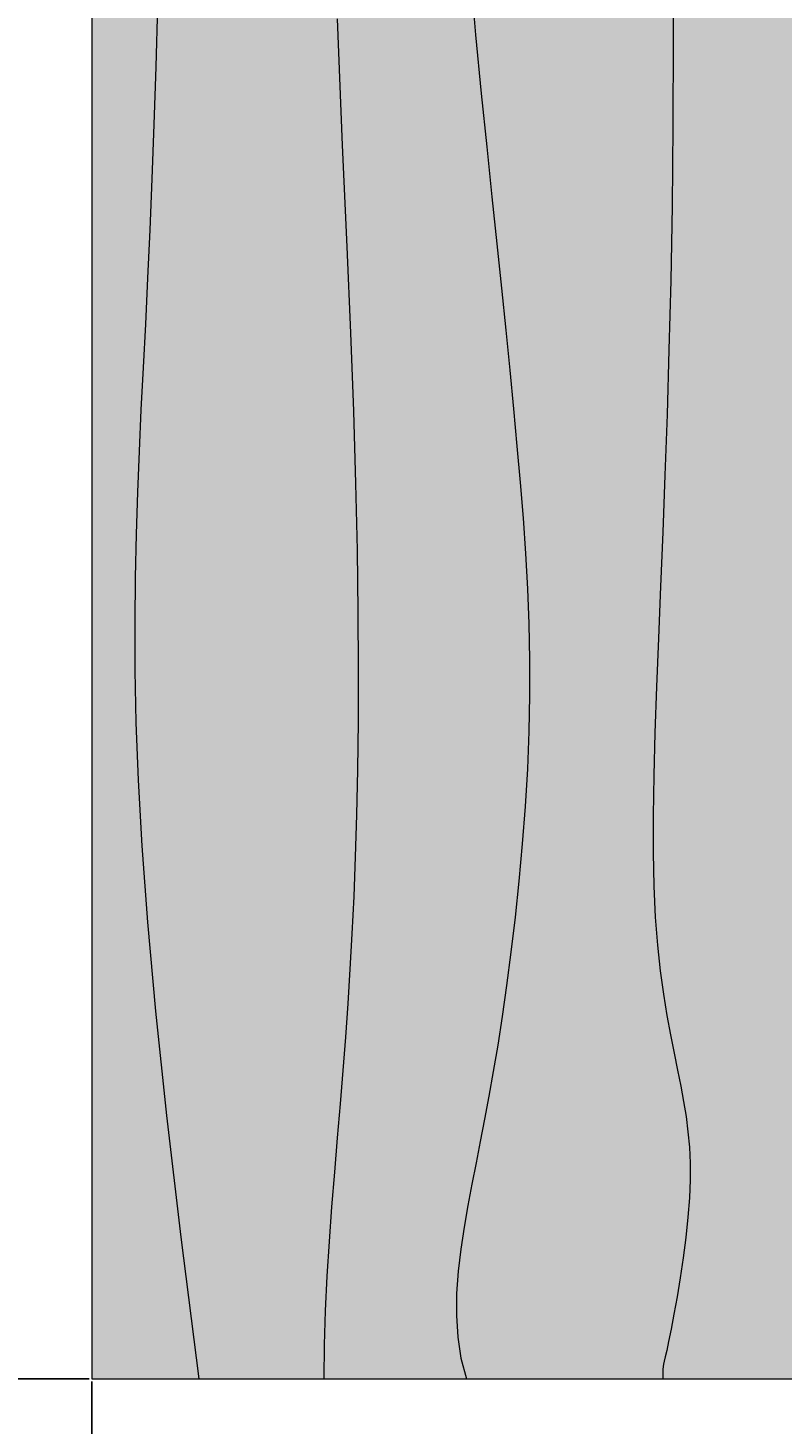
# Model space of a CAD drawing. Units: inches. Extents: x 2549 to 3108, y 1683 to 2362.
# Tile 24 of 30: x 2949 to 2966, y 2018 to 2049. Entities that reach past the tile are written whole.
import ezdxf

# ---------------------------------------------------------------- set-up
doc = ezdxf.new("R2010")
doc.units = ezdxf.units.IN
for name, color, linetype, lineweight in [('A-ANNO-DIMS', 2, 'Continuous', 18), ('A-FURN', 8, 'Continuous', 18), ('A-FURN-PATT', 9, 'Continuous', 13)]:
    doc.layers.add(name, color=color, linetype=linetype, lineweight=lineweight)
doc.layers.add('C-PKNG-VEHI-PATT', color=251, linetype='Continuous', lineweight=13, true_color=0x636466)
doc.layers.add('C-PVMT-PATT', color=9, linetype='Continuous', lineweight=13, true_color=0xc7c8ca)
doc.styles.get("Standard").update_dxf_attribs({"font": 'arial.ttf'})
doc.dimstyles.get("Standard").update_dxf_attribs({"dimtxt": 0.18, "dimasz": 0.18, "dimexe": 0.18, "dimexo": 0.0625, "dimgap": 0.09, "dimtad": 0, "dimtih": 1, "dimtoh": 1, "dimdec": 4, "dimzin": 0, "dimdsep": 46, "dimtxsty": 'Standard', "dimcen": 0.09, "dimadec": 0, "dimazin": 0, "dimtfac": 1, "dimtdec": 4, "dimtofl": 0, "dimtmove": 0, "dimatfit": 3, "dimfxl": 1, "dimtolj": 1, "dimtzin": 0, "dimarcsym": 0})

# ---------------------------------------------------------------- blocks, each defined once
blk = doc.blocks.new('Table - Rectangular Woodgrain 60 x 30 in.')
for p, q in [((60, -30), (60, 0)), ((0, -30), (60, -30))]:
    blk.add_line(p, q)
for points in [[(27.9, -16.9667), (29.9928, -16.9617), (31.9302, -16.9703), (33.7254, -16.9907), (35.3917, -17.0208), (36.9423, -17.0588), (38.3906, -17.1026), (39.7499, -17.1503), (41.0333, -17.2), (42.2519, -17.2496), (43.4073, -17.2969), (44.4986, -17.3395), (45.525, -17.375), (46.4858, -17.4012), (47.3802, -17.4156), (48.2074, -17.416), (48.9667, -17.4), (49.6583, -17.3662), (50.2872, -17.3167), (50.8595, -17.2547), (51.3812, -17.1833), (51.8584, -17.1057), (52.2971, -17.025), (52.7034, -16.9443), (53.0833, -16.8667), (53.443, -16.7951), (53.789, -16.7313), (54.128, -16.6768), (54.4666, -16.6334), (54.8115, -16.6024), (55.1693, -16.5854), (55.5465, -16.5841), (55.95, -16.6), (56.3828, -16.6337), (56.8346, -16.6823), (57.2915, -16.7418), (57.7396, -16.8084), (58.165, -16.878), (58.5539, -16.9469), (58.8924, -17.0111), (59.1666, -17.0667), (59.3679, -17.1107), (59.5078, -17.1438), (59.6032, -17.1675), (59.6708, -17.1833), (59.7275, -17.193), (59.7901, -17.1979), (59.8753, -17.1998), (60, -17.2)], [(28.2656, -21.5281), (29.884, -21.3947), (31.2, -21.2667), (32.3967, -21.1448), (33.5172, -21.0292), (34.5697, -20.9198), (35.5625, -20.8167), (36.5037, -20.7198), (37.4015, -20.6292), (38.2642, -20.5448), (39.1, -20.4667), (39.9164, -20.3951), (40.7187, -20.3313), (41.5117, -20.2768), (42.3, -20.2333), (43.0883, -20.2024), (43.8812, -20.1854), (44.6836, -20.1841), (45.5, -20.2), (46.3328, -20.234), (47.1747, -20.2844), (48.0163, -20.3488), (48.8479, -20.425), (49.66, -20.5106), (50.4429, -20.6031), (51.1872, -20.7004), (51.8833, -20.8), (52.5246, -20.8999), (53.1166, -20.9995), (53.6681, -21.0983), (54.1875, -21.1958), (54.6834, -21.2919), (55.1646, -21.3859), (55.6394, -21.4777), (56.1167, -21.5667), (56.6028, -21.6515), (57.0961, -21.7266), (57.5929, -21.7852), (58.0896, -21.8208), (58.5823, -21.8268), (59.0674, -21.7964), (59.5412, -21.723), (60, -21.6)], [(29.529, -24.4988), (32.3578, -24.3844), (34.6359, -24.284), (36.5667, -24.2), (38.3213, -24.1341), (39.9417, -24.0854), (41.437, -24.0523), (42.8167, -24.0333), (44.0901, -24.0268), (45.2667, -24.0313), (46.3557, -24.0451), (47.3667, -24.0667), (48.309, -24.0947), (49.1928, -24.1287), (50.0284, -24.168), (50.826, -24.2125), (51.5959, -24.2617), (52.3483, -24.3151), (53.0935, -24.3725), (53.8417, -24.4334), (54.6009, -24.497), (55.3699, -24.561), (56.1454, -24.6226), (56.9239, -24.6792), (57.7021, -24.7279), (58.4764, -24.7662), (59.2435, -24.7911), (60, -24.8)], [(29.2276, -28.5281), (30.6033, -28.5663), (31.8958, -28.6084), (33.1118, -28.6535), (34.2578, -28.7011), (35.3405, -28.7501), (36.3666, -28.8), (37.3443, -28.8497), (38.288, -28.8974), (39.2137, -28.9412), (40.1375, -28.9792), (41.0753, -29.0093), (42.0432, -29.0297), (43.0572, -29.0384), (44.1333, -29.0333), (45.2936, -29.0114), (46.5843, -28.9641), (48.0579, -28.8816), (49.7666, -28.7542), (51.7629, -28.5721), (54.0989, -28.3255), (56.8272, -28.0048), (60, -27.6)]]:
    blk.add_lwpolyline(points)
blk = doc.blocks.new('*D22')
at = {"layer": 'A-ANNO-DIMS', "color": 0, "lineweight": -2, "transparency": 16777216}
for p, q in [((2950.031, 2078.615), (2940.913, 2078.615)), ((2941.093, 2078.435), (2941.093, 2048.798)), ((2941.093, 2018.795), (2941.093, 2048.431)), ((2950.031, 2018.615), (2940.913, 2018.615))]:
    blk.add_line(p, q, dxfattribs=at)
at = {"layer": 'A-ANNO-DIMS', "color": 0, "transparency": 16777216}
for points in [[(2941.063, 2078.435), (2941.123, 2078.435), (2941.093, 2078.615)], [(2941.063, 2018.795), (2941.123, 2018.795), (2941.093, 2018.615)]]:
    blk.add_solid(points, dxfattribs=at)
at = {"layer": 'Defpoints', "color": 0, "transparency": 16777216}
for p in [(2950.093, 2078.615), (2941.093, 2018.615), (2950.093, 2018.615)]:
    blk.add_point(p, dxfattribs=at)
at = {"layer": 'A-ANNO-DIMS', "color": 0, "transparency": 16777216, "insert": (2941.093, 2048.615), "char_height": 0.18, "attachment_point": 5}
blk.add_mtext('\\A1;COFFEE TABLE 60', dxfattribs=at)
blk = doc.blocks.new('*D23')
at = {"layer": 'A-ANNO-DIMS', "color": 0, "lineweight": -2, "transparency": 16777216}
for p, q in [((2950.093, 2018.552), (2950.093, 2009.435)), ((2980.093, 2018.552), (2980.093, 2009.435)), ((2950.273, 2009.615), (2964.875, 2009.615)), ((2979.913, 2009.615), (2965.312, 2009.615))]:
    blk.add_line(p, q, dxfattribs=at)
at = {"layer": 'A-ANNO-DIMS', "color": 0, "transparency": 16777216}
for points in [[(2950.273, 2009.645), (2950.273, 2009.585), (2950.093, 2009.615)], [(2979.913, 2009.645), (2979.913, 2009.585), (2980.093, 2009.615)]]:
    blk.add_solid(points, dxfattribs=at)
at = {"layer": 'Defpoints', "color": 0, "transparency": 16777216}
for p in [(2950.093, 2018.615), (2980.093, 2018.615), (2980.093, 2009.615)]:
    blk.add_point(p, dxfattribs=at)
at = {"layer": 'A-ANNO-DIMS', "color": 0, "transparency": 16777216, "insert": (2965.093, 2009.615), "char_height": 0.18, "attachment_point": 5}
blk.add_mtext('\\A1;30', dxfattribs=at)
blk = doc.blocks.new('*D46')
at = {"layer": 'A-ANNO-DIMS', "color": 0, "lineweight": -2, "transparency": 16777216}
for p, q in [((2812.643, 2140.461), (2812.643, 1683.444)), ((3034.643, 2134.461), (3034.643, 1683.444)), ((2812.823, 1683.624), (2923.353, 1683.624)), ((3034.463, 1683.624), (2923.932, 1683.624))]:
    blk.add_line(p, q, dxfattribs=at)
at = {"layer": 'A-ANNO-DIMS', "color": 0, "transparency": 16777216}
for points in [[(2812.823, 1683.654), (2812.823, 1683.594), (2812.643, 1683.624)], [(3034.463, 1683.654), (3034.463, 1683.594), (3034.643, 1683.624)]]:
    blk.add_solid(points, dxfattribs=at)
at = {"layer": 'Defpoints', "color": 0, "transparency": 16777216}
for p in [(2812.643, 2140.524), (3034.643, 2134.524), (3034.643, 1683.624)]:
    blk.add_point(p, dxfattribs=at)
at = {"layer": 'A-ANNO-DIMS', "color": 0, "transparency": 16777216, "insert": (2923.643, 1683.624), "char_height": 0.18, "attachment_point": 5}
blk.add_mtext('\\A1;222', dxfattribs=at)
blk = doc.blocks.new('*D63')
at = {"layer": 'A-ANNO-DIMS', "color": 0, "lineweight": -2, "transparency": 16777216}
for p, q in [((2963.328, 2197.213), (2963.508, 2197.213)), ((2963.508, 2197.213), (2963.508, 2124.675)), ((2963.419, 2003.299), (2963.599, 2003.299)), ((2963.509, 2003.209), (2963.509, 2003.389))]:
    blk.add_line(p, q, dxfattribs=at)
at = {"layer": 'A-ANNO-DIMS', "color": 0, "transparency": 16777216}
blk.add_solid([(2963.538, 2124.675), (2963.478, 2124.675), (2963.508, 2124.495)], dxfattribs=at)
at = {"layer": 'Defpoints', "color": 0, "transparency": 16777216}
for p in [(2963.508, 2124.495), (2963.509, 2003.299)]:
    blk.add_point(p, dxfattribs=at)
at = {"layer": 'A-ANNO-DIMS', "color": 0, "transparency": 16777216, "insert": (2962.654, 2197.213), "char_height": 0.18, "attachment_point": 5}
blk.add_mtext('\\A1;2X R121.2', dxfattribs=at)

msp = doc.modelspace()

# ---------------------------------------------------------------- hatches: boundary and pattern name
at = {"layer": 'A-FURN-PATT', "transparency": 33554684}
h = msp.add_hatch(color=256, dxfattribs=at)
h.dxf.hatch_style = 1
h.paths.add_polyline_path([(2951.6587, 2056.0021), (2951.6557, 2058.2435), (2951.6347, 2060.9396), (2951.5919, 2064.2076), (2951.5233, 2068.1646), (2951.425, 2072.9279), (2951.2931, 2078.6146), (2950.0931, 2078.6146), (2950.0931, 2018.6146), (2952.4931, 2018.6146), (2952.0883, 2021.7874), (2951.7676, 2024.5157), (2951.521, 2026.8517), (2951.3389, 2028.848), (2951.2115, 2030.5567), (2951.129, 2032.0303), (2951.0817, 2033.321), (2951.0598, 2034.4813), (2951.0547, 2035.5574), (2951.0634, 2036.5714), (2951.0838, 2037.5393), (2951.1139, 2038.4771), (2951.1519, 2039.4009), (2951.1957, 2040.3266), (2951.2434, 2041.2703), (2951.2931, 2042.248), (2951.343, 2043.2741), (2951.392, 2044.3568), (2951.4396, 2045.5028), (2951.4847, 2046.7188), (2951.5268, 2048.0113), (2951.565, 2049.387), (2951.5984, 2050.8526), (2951.6264, 2052.4146), (2951.6476, 2054.0982)])
h.paths.add_polyline_path([(2955.3325, 2057.2097), (2955.19, 2062.912), (2955.0427, 2069.9791), (2954.8931, 2078.6146), (2951.2931, 2078.6146), (2951.425, 2072.9279), (2951.5233, 2068.1646), (2951.5919, 2064.2076), (2951.6347, 2060.9396), (2951.6557, 2058.2435), (2951.6587, 2056.0021), (2951.6476, 2054.0982), (2951.6264, 2052.4146), (2951.5984, 2050.8526), (2951.565, 2049.387), (2951.5268, 2048.0113), (2951.4847, 2046.7188), (2951.4396, 2045.5028), (2951.392, 2044.3568), (2951.343, 2043.2741), (2951.2931, 2042.248), (2951.2434, 2041.2703), (2951.1957, 2040.3266), (2951.1519, 2039.4009), (2951.1139, 2038.4771), (2951.0838, 2037.5393), (2951.0634, 2036.5714), (2951.0547, 2035.5574), (2951.0598, 2034.4813), (2951.0817, 2033.321), (2951.129, 2032.0303), (2951.2115, 2030.5567), (2951.3389, 2028.848), (2951.521, 2026.8517), (2951.7676, 2024.5157), (2952.0883, 2021.7874), (2952.4931, 2018.6146), (2955.2931, 2018.6146), (2955.302, 2019.3711), (2955.3269, 2020.1382), (2955.3652, 2020.9125), (2955.4139, 2021.6907), (2955.4705, 2022.4692), (2955.5321, 2023.2447), (2955.5961, 2024.0137), (2955.6597, 2024.7729), (2955.7206, 2025.5211), (2955.778, 2026.2663), (2955.8314, 2027.0187), (2955.8806, 2027.7886), (2955.9251, 2028.5862), (2955.9644, 2029.4218), (2955.9984, 2030.3056), (2956.0264, 2031.2479), (2956.048, 2032.2589), (2956.0618, 2033.3479), (2956.0663, 2034.5245), (2956.0598, 2035.7979), (2956.0408, 2037.1776), (2956.0077, 2038.6729), (2955.959, 2040.2933), (2955.8931, 2042.0479), (2955.8091, 2043.9787), (2955.7087, 2046.2568), (2955.5943, 2049.0856), (2955.4681, 2052.6688)])
h.paths.add_polyline_path([(2958.1396, 2059.1978), (2957.992, 2064.2052), (2957.843, 2070.6048), (2957.6931, 2078.6146), (2954.8931, 2078.6146), (2955.0427, 2069.9791), (2955.19, 2062.912), (2955.3325, 2057.2097), (2955.4681, 2052.6688), (2955.5943, 2049.0856), (2955.7087, 2046.2568), (2955.8091, 2043.9787), (2955.8931, 2042.0479), (2955.959, 2040.2933), (2956.0077, 2038.6729), (2956.0408, 2037.1776), (2956.0598, 2035.7979), (2956.0663, 2034.5245), (2956.0618, 2033.3479), (2956.048, 2032.2589), (2956.0264, 2031.2479), (2955.9984, 2030.3056), (2955.9644, 2029.4218), (2955.9251, 2028.5862), (2955.8806, 2027.7886), (2955.8314, 2027.0187), (2955.778, 2026.2663), (2955.7206, 2025.5211), (2955.6597, 2024.7729), (2955.5961, 2024.0137), (2955.5321, 2023.2447), (2955.4705, 2022.4692), (2955.4139, 2021.6907), (2955.3652, 2020.9125), (2955.3269, 2020.1382), (2955.302, 2019.3711), (2955.2931, 2018.6146), (2958.4931, 2018.6146), (2958.3701, 2019.0734), (2958.2967, 2019.5472), (2958.2663, 2020.0323), (2958.2723, 2020.525), (2958.3079, 2021.0217), (2958.3665, 2021.5185), (2958.4416, 2022.0118), (2958.5264, 2022.4979), (2958.6154, 2022.9752), (2958.7072, 2023.45), (2958.8012, 2023.9312), (2958.8973, 2024.4271), (2958.9948, 2024.9465), (2959.0936, 2025.498), (2959.1932, 2026.09), (2959.2931, 2026.7313), (2959.3927, 2027.4274), (2959.49, 2028.1717), (2959.5825, 2028.9546), (2959.6681, 2029.7667), (2959.7443, 2030.5983), (2959.8087, 2031.4399), (2959.8591, 2032.2818), (2959.8931, 2033.1146), (2959.909, 2033.931), (2959.9077, 2034.7334), (2959.8907, 2035.5263), (2959.8598, 2036.3146), (2959.8163, 2037.1029), (2959.7618, 2037.8959), (2959.698, 2038.6982), (2959.6264, 2039.5146), (2959.5483, 2040.3504), (2959.4639, 2041.2131), (2959.3733, 2042.1109), (2959.2764, 2043.0521), (2959.1733, 2044.0449), (2959.0639, 2045.0974), (2958.9483, 2046.2179), (2958.8264, 2047.4146), (2958.6984, 2048.7306), (2958.565, 2050.349), (2958.4268, 2052.4877), (2958.2848, 2055.3646)])
h.paths.add_polyline_path([(2963.0634, 2055.4818), (2962.9958, 2058.2679), (2962.8973, 2061.4021), (2962.7628, 2064.9441), (2962.5874, 2068.9537), (2962.3658, 2073.4906), (2962.0931, 2078.6146), (2957.6931, 2078.6146), (2957.843, 2070.6048), (2957.992, 2064.2052), (2958.1396, 2059.1978), (2958.2848, 2055.3646), (2958.4268, 2052.4877), (2958.565, 2050.349), (2958.6984, 2048.7306), (2958.8264, 2047.4146), (2958.9483, 2046.2179), (2959.0639, 2045.0974), (2959.1733, 2044.0449), (2959.2764, 2043.0521), (2959.3733, 2042.1109), (2959.4639, 2041.2131), (2959.5483, 2040.3504), (2959.6264, 2039.5146), (2959.698, 2038.6982), (2959.7618, 2037.8959), (2959.8163, 2037.1029), (2959.8598, 2036.3146), (2959.8907, 2035.5263), (2959.9077, 2034.7334), (2959.909, 2033.931), (2959.8931, 2033.1146), (2959.8591, 2032.2818), (2959.8087, 2031.4399), (2959.7443, 2030.5983), (2959.6681, 2029.7667), (2959.5825, 2028.9546), (2959.49, 2028.1717), (2959.3927, 2027.4274), (2959.2931, 2026.7313), (2959.1932, 2026.09), (2959.0936, 2025.498), (2958.9948, 2024.9465), (2958.8973, 2024.4271), (2958.8012, 2023.9312), (2958.7072, 2023.45), (2958.6154, 2022.9752), (2958.5264, 2022.4979), (2958.4416, 2022.0118), (2958.3665, 2021.5185), (2958.3079, 2021.0217), (2958.2723, 2020.525), (2958.2663, 2020.0323), (2958.2967, 2019.5472), (2958.3701, 2019.0734), (2958.4931, 2018.6146), (2962.8931, 2018.6146), (2962.8935, 2018.8741), (2962.9256, 2019.0114), (2962.9493, 2019.1068), (2962.9824, 2019.2467), (2963.0264, 2019.448), (2963.082, 2019.7222), (2963.1462, 2020.0607), (2963.2151, 2020.4496), (2963.2847, 2020.875), (2963.3513, 2021.3231), (2963.4108, 2021.78), (2963.4594, 2022.2318), (2963.4931, 2022.6646), (2963.509, 2023.0681), (2963.5077, 2023.4453), (2963.4907, 2023.8031), (2963.4597, 2024.148), (2963.4163, 2024.4866), (2963.3618, 2024.8256), (2963.298, 2025.1716), (2963.2264, 2025.5313), (2963.1488, 2025.9112), (2963.0681, 2026.3175), (2962.9874, 2026.7562), (2962.9098, 2027.2334), (2962.8384, 2027.7551), (2962.7764, 2028.3274), (2962.7269, 2028.9563), (2962.6931, 2029.6479), (2962.6771, 2030.4072), (2962.6775, 2031.2344), (2962.6919, 2032.1288), (2962.7181, 2033.0896), (2962.7536, 2034.116), (2962.7962, 2035.2073), (2962.8435, 2036.3627), (2962.8931, 2037.5813), (2962.9428, 2038.8647), (2962.9905, 2040.224), (2963.0343, 2041.6723), (2963.0723, 2043.2229), (2963.1024, 2044.8892), (2963.1228, 2046.6844), (2963.1314, 2048.6218), (2963.1264, 2050.7146), (2963.1053, 2052.9839)])
h.paths.add_polyline_path([(2967.0608, 2068.9933), (2967.1609, 2073.4299), (2967.2931, 2078.6146), (2962.0931, 2078.6146), (2962.3658, 2073.4906), (2962.5874, 2068.9537), (2962.7628, 2064.9441), (2962.8973, 2061.4021), (2962.9958, 2058.2679), (2963.0634, 2055.4818), (2963.1053, 2052.9839), (2963.1264, 2050.7146), (2963.1314, 2048.6218), (2963.1228, 2046.6844), (2963.1024, 2044.8892), (2963.0723, 2043.2229), (2963.0343, 2041.6723), (2962.9905, 2040.224), (2962.9428, 2038.8647), (2962.8931, 2037.5813), (2962.8435, 2036.3627), (2962.7962, 2035.2073), (2962.7536, 2034.116), (2962.7181, 2033.0896), (2962.6919, 2032.1288), (2962.6775, 2031.2344), (2962.6771, 2030.4072), (2962.6931, 2029.6479), (2962.7269, 2028.9563), (2962.7764, 2028.3274), (2962.8384, 2027.7551), (2962.9098, 2027.2334), (2962.9874, 2026.7562), (2963.0681, 2026.3175), (2963.1488, 2025.9112), (2963.2264, 2025.5313), (2963.298, 2025.1716), (2963.3618, 2024.8256), (2963.4163, 2024.4866), (2963.4597, 2024.148), (2963.4907, 2023.8031), (2963.5077, 2023.4453), (2963.509, 2023.0681), (2963.4931, 2022.6646), (2963.4594, 2022.2318), (2963.4108, 2021.78), (2963.3513, 2021.3231), (2963.2847, 2020.875), (2963.2151, 2020.4496), (2963.1462, 2020.0607), (2963.082, 2019.7222), (2963.0264, 2019.448), (2962.9824, 2019.2467), (2962.9493, 2019.1068), (2962.9256, 2019.0114), (2962.9098, 2018.9438), (2962.9001, 2018.8871), (2962.8952, 2018.8245), (2962.8933, 2018.7393), (2962.8931, 2018.6146), (2966.4931, 2018.6146), (2966.7749, 2019.8457), (2967.0223, 2020.8601), (2967.2384, 2021.6895), (2967.4264, 2022.3657), (2967.5894, 2022.9204), (2967.7306, 2023.3853), (2967.853, 2023.7923), (2967.9598, 2024.173), (2968.0534, 2024.5532), (2968.1337, 2024.9351), (2968.2, 2025.3148), (2968.2514, 2025.6886), (2968.2872, 2026.0526), (2968.3066, 2026.403), (2968.3088, 2026.7361), (2968.2931, 2027.048), (2968.259, 2027.3358), (2968.2077, 2027.6011), (2968.1407, 2027.846), (2968.0598, 2028.073), (2967.9663, 2028.2843), (2967.8618, 2028.4823), (2967.748, 2028.6694), (2967.6264, 2028.8479), (2967.4987, 2029.0209), (2967.367, 2029.1938), (2967.2338, 2029.3729), (2967.1014, 2029.5646), (2966.9721, 2029.775), (2966.8483, 2030.0104), (2966.7323, 2030.2771), (2966.6264, 2030.5813), (2966.5327, 2030.9288), (2966.4514, 2031.324), (2966.3827, 2031.7707), (2966.3264, 2032.273), (2966.2827, 2032.8345), (2966.2514, 2033.4594), (2966.2327, 2034.1515), (2966.2264, 2034.9146), (2966.2324, 2035.7506), (2966.2493, 2036.6521), (2966.2757, 2037.6099), (2966.3098, 2038.6146), (2966.3501, 2039.6568), (2966.3952, 2040.7271), (2966.4434, 2041.8162), (2966.4931, 2042.9146), (2966.543, 2044.0176), (2966.5921, 2045.1386), (2966.6396, 2046.2955), (2966.6848, 2047.5063), (2966.7268, 2048.789), (2966.765, 2050.1615), (2966.7984, 2051.6418), (2966.8264, 2053.248), (2966.8492, 2055.0092), (2966.8712, 2057.0006), (2966.8979, 2059.3083), (2966.9348, 2062.0188), (2966.9872, 2065.2183)])
h.paths.add_polyline_path([(2971.0073, 2072.0387), (2970.8931, 2078.6146), (2967.2931, 2078.6146), (2967.1609, 2073.4299), (2967.0608, 2068.9933), (2966.9872, 2065.2183), (2966.9348, 2062.0188), (2966.8979, 2059.3083), (2966.8712, 2057.0006), (2966.8492, 2055.0092), (2966.8264, 2053.248), (2966.7984, 2051.6418), (2966.765, 2050.1615), (2966.7268, 2048.789), (2966.6848, 2047.5063), (2966.6396, 2046.2955), (2966.5921, 2045.1386), (2966.543, 2044.0176), (2966.4931, 2042.9146), (2966.4434, 2041.8162), (2966.3952, 2040.7271), (2966.3501, 2039.6568), (2966.3098, 2038.6146), (2966.2757, 2037.6099), (2966.2493, 2036.6521), (2966.2324, 2035.7506), (2966.2264, 2034.9146), (2966.2327, 2034.1515), (2966.2514, 2033.4594), (2966.2827, 2032.8345), (2966.3264, 2032.273), (2966.3827, 2031.7707), (2966.4514, 2031.324), (2966.5327, 2030.9288), (2966.6264, 2030.5813), (2966.7323, 2030.2771), (2966.8483, 2030.0104), (2966.9721, 2029.775), (2967.1014, 2029.5646), (2967.2338, 2029.3729), (2967.367, 2029.1938), (2967.4987, 2029.0209), (2967.6264, 2028.8479), (2967.748, 2028.6694), (2967.8618, 2028.4823), (2967.9663, 2028.2843), (2968.0598, 2028.073), (2968.1407, 2027.846), (2968.2077, 2027.6011), (2968.259, 2027.3358), (2968.2931, 2027.048), (2968.3088, 2026.7361), (2968.3066, 2026.403), (2968.2872, 2026.0526), (2968.2514, 2025.6886), (2968.2, 2025.3148), (2968.1337, 2024.9351), (2968.0534, 2024.5532), (2967.9598, 2024.173), (2967.853, 2023.7923), (2967.7306, 2023.3853), (2967.5894, 2022.9204), (2967.4264, 2022.3657), (2967.2384, 2021.6895), (2967.0223, 2020.8601), (2966.7749, 2019.8457), (2966.4931, 2018.6146), (2970.0931, 2018.6146), (2970.5775, 2020.6947), (2971.1181, 2022.524), (2971.6962, 2024.1236), (2972.2931, 2025.5146), (2972.89, 2026.7181), (2973.4681, 2027.7552), (2974.0087, 2028.647), (2974.4931, 2029.4146), (2974.9065, 2030.0774), (2975.2504, 2030.6485), (2975.5302, 2031.139), (2975.7514, 2031.5604), (2975.9195, 2031.924), (2976.04, 2032.2412), (2976.1182, 2032.5231), (2976.1598, 2032.7813), (2976.1697, 2033.0246), (2976.1514, 2033.2532), (2976.1082, 2033.4645), (2976.0431, 2033.6563), (2975.9592, 2033.8262), (2975.8598, 2033.9719), (2975.7478, 2034.091), (2975.6264, 2034.1813), (2975.4975, 2034.241), (2975.3577, 2034.2719), (2975.2022, 2034.2762), (2975.0264, 2034.2563), (2974.8256, 2034.2145), (2974.5952, 2034.1532), (2974.3303, 2034.0746), (2974.0264, 2033.9813), (2973.6814, 2033.8758), (2973.3035, 2033.7625), (2972.9038, 2033.6461), (2972.4931, 2033.5313), (2972.0824, 2033.4227), (2971.6827, 2033.325), (2971.3048, 2033.243), (2970.9598, 2033.1813), (2970.656, 2033.1437), (2970.392, 2033.1302), (2970.1641, 2033.1403), (2969.9681, 2033.173), (2969.8002, 2033.2275), (2969.6566, 2033.3032), (2969.5333, 2033.3991), (2969.4264, 2033.5146), (2969.3328, 2033.6498), (2969.2525, 2033.8084), (2969.1862, 2033.9951), (2969.1348, 2034.2146), (2969.0989, 2034.4716), (2969.0795, 2034.7709), (2969.0773, 2035.117), (2969.0931, 2035.5146), (2969.1271, 2035.9681), (2969.1775, 2036.4802), (2969.2419, 2037.0533), (2969.3181, 2037.6896), (2969.4036, 2038.3916), (2969.4962, 2039.1615), (2969.5935, 2040.0017), (2969.6931, 2040.9146), (2969.7932, 2041.9018), (2969.8941, 2042.962), (2969.9966, 2044.0933), (2970.1014, 2045.2938), (2970.2094, 2046.5614), (2970.3212, 2047.8943), (2970.4378, 2049.2905), (2970.5598, 2050.748), (2970.6862, 2052.2926), (2970.8087, 2054.0615), (2970.9172, 2056.2194), (2971.0014, 2058.9313), (2971.0513, 2062.3619), (2971.0566, 2066.6761)])
h.paths.add_polyline_path([(2977.5454, 2065.9056), (2977.6243, 2069.5844), (2977.6751, 2073.7991), (2977.6931, 2078.6146), (2970.8931, 2078.6146), (2971.0073, 2072.0387), (2971.0566, 2066.6761), (2971.0513, 2062.3619), (2971.0014, 2058.9313), (2970.9172, 2056.2194), (2970.8087, 2054.0615), (2970.6862, 2052.2926), (2970.5598, 2050.748), (2970.4378, 2049.2905), (2970.3212, 2047.8943), (2970.2094, 2046.5614), (2970.1014, 2045.2938), (2969.9966, 2044.0933), (2969.8941, 2042.962), (2969.7932, 2041.9018), (2969.6931, 2040.9146), (2969.5935, 2040.0017), (2969.4962, 2039.1615), (2969.4036, 2038.3916), (2969.3181, 2037.6896), (2969.2419, 2037.0533), (2969.1775, 2036.4802), (2969.1271, 2035.9681), (2969.0931, 2035.5146), (2969.0773, 2035.117), (2969.0795, 2034.7709), (2969.0989, 2034.4716), (2969.1348, 2034.2146), (2969.1862, 2033.9951), (2969.2525, 2033.8084), (2969.3328, 2033.6498), (2969.4264, 2033.5146), (2969.5333, 2033.3991), (2969.6566, 2033.3032), (2969.8002, 2033.2275), (2969.9681, 2033.173), (2970.1641, 2033.1403), (2970.392, 2033.1302), (2970.656, 2033.1437), (2970.9598, 2033.1813), (2971.3048, 2033.243), (2971.6827, 2033.325), (2972.0824, 2033.4227), (2972.4931, 2033.5313), (2972.9038, 2033.6461), (2973.3035, 2033.7625), (2973.6814, 2033.8758), (2974.0264, 2033.9813), (2974.3303, 2034.0746), (2974.5952, 2034.1532), (2974.8256, 2034.2145), (2975.1314, 2034.2781), (2975.4354, 2034.2697), (2975.6264, 2034.1813), (2975.7478, 2034.091), (2975.8598, 2033.9719), (2975.9592, 2033.8262), (2976.0431, 2033.6563), (2976.1082, 2033.4645), (2976.1514, 2033.2532), (2976.1697, 2033.0246), (2976.1598, 2032.7813), (2976.1182, 2032.5231), (2976.04, 2032.2412), (2975.9195, 2031.924), (2975.7514, 2031.5604), (2975.5302, 2031.139), (2975.2504, 2030.6485), (2974.9065, 2030.0774), (2974.4931, 2029.4146), (2974.0087, 2028.647), (2973.4681, 2027.7552), (2972.89, 2026.7181), (2972.2931, 2025.5146), (2971.6962, 2024.1236), (2971.1181, 2022.524), (2970.5775, 2020.6947), (2970.0931, 2018.6146), (2976.8931, 2018.6146), (2977.043, 2020.5019), (2977.192, 2022.3313), (2977.3396, 2024.092), (2977.4848, 2025.773), (2977.6268, 2027.3633), (2977.765, 2028.8521), (2977.8984, 2030.2284), (2978.0264, 2031.4813), (2978.1482, 2032.6032), (2978.2629, 2033.6006), (2978.3698, 2034.483), (2978.4681, 2035.2604), (2978.557, 2035.9425), (2978.6358, 2036.5391), (2978.7036, 2037.0599), (2978.7598, 2037.5146), (2978.8035, 2037.9123), (2978.8348, 2038.2584), (2978.8535, 2038.5576), (2978.8598, 2038.8146), (2978.8535, 2039.0342), (2978.8348, 2039.2209), (2978.8035, 2039.3795), (2978.7598, 2039.5146), (2978.7038, 2039.6302), (2978.6368, 2039.7271), (2978.5605, 2039.8052), (2978.4764, 2039.8646), (2978.3861, 2039.9052), (2978.291, 2039.9271), (2978.1928, 2039.9302), (2978.0931, 2039.9146), (2977.993, 2039.8809), (2977.8921, 2039.8323), (2977.7896, 2039.7728), (2977.6848, 2039.7063), (2977.5003, 2039.5872), (2977.2813, 2039.4666), (2977.0307, 2039.3815), (2976.7627, 2039.3587), (2976.5032, 2039.4189), (2976.3323, 2039.5382), (2976.2264, 2039.648), (2976.1329, 2039.7907), (2976.0535, 2039.9771), (2975.9897, 2040.2198), (2975.9431, 2040.5313), (2975.9152, 2040.924), (2975.9077, 2041.4105), (2975.922, 2042.0032), (2975.9597, 2042.7146), (2976.0217, 2043.5556), (2976.1056, 2044.5297), (2976.2082, 2045.639), (2976.3264, 2046.8855), (2976.4571, 2048.2709), (2976.5973, 2049.7974), (2976.7436, 2051.4669), (2976.8931, 2053.2813), (2977.0423, 2055.253), (2977.1868, 2057.4365), (2977.322, 2059.8965), (2977.4431, 2062.6979)])
h.paths.add_polyline_path([(2980.0931, 2078.6146), (2977.6931, 2078.6146), (2977.6751, 2073.7991), (2977.6243, 2069.5844), (2977.5454, 2065.9056), (2977.4431, 2062.6979), (2977.322, 2059.8965), (2977.1868, 2057.4365), (2977.0423, 2055.253), (2976.8931, 2053.2813), (2976.7436, 2051.4669), (2976.5973, 2049.7974), (2976.4571, 2048.2709), (2976.3264, 2046.8855), (2976.2082, 2045.639), (2976.1056, 2044.5297), (2976.0217, 2043.5556), (2975.9597, 2042.7146), (2975.922, 2042.0032), (2975.9077, 2041.4105), (2975.9152, 2040.924), (2975.9431, 2040.5313), (2975.9897, 2040.2198), (2976.0535, 2039.9771), (2976.1329, 2039.7907), (2976.2264, 2039.648), (2976.3323, 2039.5382), (2976.4483, 2039.4573), (2976.5721, 2039.403), (2976.7014, 2039.373), (2976.8338, 2039.3648), (2976.967, 2039.3761), (2977.0987, 2039.4046), (2977.2264, 2039.448), (2977.3484, 2039.5036), (2977.465, 2039.5678), (2977.5768, 2039.6366), (2977.7721, 2039.7626), (2977.9521, 2039.8671), (2978.144, 2039.9317), (2978.3409, 2039.9255), (2978.5228, 2039.8437), (2978.6765, 2039.6863), (2978.7598, 2039.5146), (2978.8035, 2039.3795), (2978.8348, 2039.2209), (2978.8535, 2039.0342), (2978.8598, 2038.8146), (2978.8535, 2038.5576), (2978.8348, 2038.2584), (2978.8035, 2037.9123), (2978.7598, 2037.5146), (2978.7036, 2037.0599), (2978.6358, 2036.5391), (2978.557, 2035.9425), (2978.4681, 2035.2604), (2978.3698, 2034.483), (2978.2629, 2033.6006), (2978.1482, 2032.6032), (2978.0264, 2031.4813), (2977.8984, 2030.2284), (2977.765, 2028.8521), (2977.6268, 2027.3633), (2977.4848, 2025.773), (2977.3396, 2024.092), (2977.192, 2022.3313), (2977.043, 2020.5019), (2976.8931, 2018.6146), (2980.0931, 2018.6146)])
at = {"layer": 'C-PKNG-VEHI-PATT'}
h = msp.add_hatch(color=256, dxfattribs=at)
h.dxf.hatch_style = 1
edge = h.paths.add_edge_path()
edge.add_ellipse((2935.7258, 1791.964), major_axis=(-50.66, 0), ratio=0.8423039, start_angle=248.16505, end_angle=265.72258)
edge.add_line((2938.911, 1834.5507), (2925.8653, 1834.5507))
edge.add_ellipse((2929.0505, 1791.964), major_axis=(50.66, 0), ratio=0.8423039, start_angle=94.27742, end_angle=111.83495)
edge.add_line((2912.8508, 1832.3947), (2914.2044, 1822.2495))
edge.add_ellipse((2930.6538, 1783.1023), major_axis=(-49.3014, 0), ratio=0.8423039, start_angle=-85.12993, end_angle=-67.20809, ccw=False)
edge.add_line((2927.1247, 1824.5225), (2937.6516, 1824.5225))
edge.add_ellipse((2934.1225, 1783.1023), major_axis=(49.3014, 0), ratio=0.8423039, start_angle=67.20809, end_angle=85.12993, ccw=False)
edge.add_line((2950.5719, 1822.2495), (2951.9255, 1832.3947))
edge = h.paths.add_edge_path()
edge.add_ellipse((2903.4793, 1857.3351), major_axis=(-34.7979, 0), ratio=0.8423039, start_angle=180, end_angle=209.43857)
edge.add_ellipse((2961.297, 1857.3351), major_axis=(34.7979, 0), ratio=0.8423039, start_angle=150.56143, end_angle=180)
edge.add_line((2926.4991, 1857.3351), (2926.4991, 1843.7609))
edge.add_ellipse((2924.1251, 1844.3143), major_axis=(-0.2209, 3.9278), ratio=0.6038336, start_angle=89.00201, end_angle=253.65741, ccw=False)
edge.add_line((2921.7512, 1844.2222), (2921.7512, 1853.3975))
edge.add_line((2921.7512, 1853.3975), (2925.269, 1855.8484))
edge.add_ellipse((2925.4782, 1855.4931), major_axis=(0.4584, 0), ratio=0.8423039, start_angle=90, end_angle=134.48021, ccw=False)
edge.add_line((2925.4782, 1855.8792), (2926.4991, 1855.8792))
edge.add_line((2926.4991, 1855.8792), (2926.4991, 1857.3351))
edge.add_ellipse((2961.297, 1857.3351), major_axis=(34.7979, 0), ratio=0.8423039, start_angle=150.56143, end_angle=180, ccw=False)
edge.add_line((2932.3882, 1873.6501), (2932.3882, 1875.7801))
edge.add_ellipse((2932.3882, 1875.3939), major_axis=(0.4584, 0), ratio=0.8423039, start_angle=90, end_angle=127.93313)
edge.add_line((2932.1366, 1875.7167), (2928.5915, 1873.7564))
edge.add_ellipse((2899.9271, 2002.4692), major_axis=(155.4756, 0), ratio=0.84230387, start_angle=-80.743434, end_angle=-77.445067, ccw=False)
edge.add_ellipse((2949.4402, 1715.2151), major_axis=(-189.1422, 0), ratio=0.84230387, start_angle=-79.790461, end_angle=-77.555373)
edge.add_ellipse((3300.3614, 1852.5642), major_axis=(-386.1662, 0), ratio=0.84230387, start_angle=-2.863715, end_angle=2.198541)
edge.add_ellipse((2929.0505, 1792.5159), major_axis=(-55.6192, 0), ratio=0.8423039, start_angle=-85.91759, end_angle=-72.28005, ccw=False)
edge.add_line((2925.7129, 1839.2798), (2939.0634, 1839.2798))
edge.add_ellipse((2935.7258, 1792.5159), major_axis=(55.6192, 0), ratio=0.8423039, start_angle=72.28005, end_angle=85.91759, ccw=False)
edge.add_ellipse((2564.4149, 1852.5642), major_axis=(-386.1662, 0), ratio=0.84230387, start_angle=177.801459, end_angle=182.863715)
edge.add_ellipse((2915.3361, 1715.2151), major_axis=(189.1422, 0), ratio=0.84230387, start_angle=77.555373, end_angle=79.790461)
edge.add_ellipse((2964.8492, 2002.4692), major_axis=(-155.4756, 0), ratio=0.84230387, start_angle=77.445067, end_angle=80.743434, ccw=False)
edge.add_line((2936.1848, 1873.7564), (2932.6397, 1875.7167))
edge.add_ellipse((2932.3882, 1875.3939), major_axis=(0.4584, 0), ratio=0.8423039, start_angle=52.06687, end_angle=90)
edge.add_line((2932.3882, 1875.7801), (2932.3882, 1873.6501))
edge.add_ellipse((2903.4793, 1857.3351), major_axis=(-34.7979, 0), ratio=0.8423039, start_angle=180, end_angle=209.43857, ccw=False)
edge.add_line((2938.2772, 1857.3351), (2938.2772, 1855.8792))
edge.add_line((2938.2772, 1855.8792), (2939.4059, 1855.8792))
edge.add_ellipse((2939.2981, 1855.4931), major_axis=(-0.4584, 0), ratio=0.8423039, start_angle=225.51979, end_angle=270, ccw=False)
edge.add_line((2939.5903, 1855.7906), (2943.0251, 1853.3975))
edge.add_line((2943.0251, 1853.3975), (2943.0251, 1844.2222))
edge.add_ellipse((2940.6512, 1844.3143), major_axis=(0.2209, 3.9278), ratio=0.6038336, start_angle=106.34259, end_angle=270.99799, ccw=False)
edge.add_line((2938.2772, 1843.7609), (2938.2772, 1857.3351))
edge = h.paths.add_edge_path()
edge.add_ellipse((2932.3882, 1865.1973), major_axis=(91.081, 0), ratio=0.8423039, start_angle=256.401865, end_angle=283.598135, ccw=False)
edge.add_line((2914.2044, 1790.0239), (2914.2044, 1778.3622))
edge.add_ellipse((2932.3882, 1853.5356), major_axis=(91.081, 0), ratio=0.8423039, start_angle=256.401865, end_angle=283.598135)
edge.add_line((2950.5719, 1778.3622), (2950.5719, 1790.0239))
edge = h.paths.add_edge_path()
edge.add_ellipse((2948.7383, 1772.3145), major_axis=(1.8336, 0), ratio=0.8423039, start_angle=0, end_angle=90)
edge.add_line((2948.7383, 1773.859), (2916.038, 1773.859))
edge.add_ellipse((2916.038, 1772.3145), major_axis=(1.8336, 0), ratio=0.8423039, start_angle=90, end_angle=180)
edge.add_line((2914.2044, 1772.3145), (2914.2044, 1760.2558))
edge.add_line((2914.2044, 1760.2558), (2950.5719, 1760.2558))
edge.add_line((2950.5719, 1760.2558), (2950.5719, 1772.3145))
h.paths.add_polyline_path([(2748.8496, 2101.6383), (2798.148, 2101.6383), (2798.148, 2111.4248), (2748.8496, 2111.4248)], flags=9)
h.paths.add_polyline_path([(2685.2081, 2101.489), (2719.3253, 2101.489), (2719.3253, 2111.2819), (2685.2081, 2111.2819)], flags=9)
h.paths.add_polyline_path([(2814.6852, 1907.1328), (2847.8384, 1907.1328), (2847.8384, 1916.9258), (2814.6852, 1916.9258)], flags=9)
h.paths.add_polyline_path([(2814.3906, 1835.5864), (2848.0172, 1835.5864), (2848.0172, 1845.3794), (2814.3906, 1845.3794)], flags=9)
h.paths.add_polyline_path([(2800.5245, 1759.1674), (2853.7435, 1759.1674), (2853.7435, 1768.954), (2800.5245, 1768.954)], flags=9)
h.paths.add_polyline_path([(2972.4611, 1807.3305), (3015.3943, 1807.3305), (3015.3943, 1817.117), (2972.4611, 1817.117)], flags=9)
h.paths.add_polyline_path([(2902.3327, 1888.6731), (2937.9131, 1888.6731), (2937.9131, 1898.4661), (2902.3327, 1898.4661)], flags=9)
h.paths.add_polyline_path([(2712.1779, 1878.9039), (2754.1257, 1878.9039), (2754.1257, 1888.6904), (2712.1779, 1888.6904)], flags=9)
h.paths.add_polyline_path([(2614.0056, 2012.812), (2650.0251, 2012.812), (2650.0251, 2022.4371), (2614.0056, 2022.4371)], flags=9)
h.paths.add_polyline_path([(2713.3129, 2003.1645), (2747.4237, 2003.1645), (2747.4237, 2012.951), (2713.3129, 2012.951)], flags=9)
h.paths.add_polyline_path([(2950.1379, 2001.6934), (2982.2992, 2001.6934), (2982.2992, 2011.48), (2950.1379, 2011.48)], flags=9)
h.paths.add_polyline_path([(2940.864, 2238.5537), (2997.5066, 2238.5537), (2997.5066, 2248.3466), (2940.864, 2248.3466)], flags=9)
h.paths.add_polyline_path([(2821.5457, 2202.8348), (2855.663, 2202.8348), (2855.663, 2212.6278), (2821.5457, 2212.6278)], flags=9)
h.paths.add_polyline_path([(2661.8026, 2238.6249), (2718.4451, 2238.6249), (2718.4451, 2248.4179), (2661.8026, 2248.4179)], flags=9)
at = {"layer": 'C-PVMT-PATT'}
h = msp.add_hatch(color=256, dxfattribs=at)
h.dxf.hatch_style = 1
h.paths.add_polyline_path([(3067.6427, 2305.5237), (2605.6427, 2305.5237), (2605.6427, 2074.5237), (2629.6427, 2074.5237), (2629.6427, 2281.5237), (3043.6427, 2281.5237), (3043.6427, 1885.5237), (3043.6427, 1872.8745), (3031.1672, 1872.8745), (3031.1672, 1862.5731), (2995.8054, 1862.5731), (2995.8054, 1872.8745), (2983.1752, 1872.8745), (2983.1752, 1885.5237), (2881.6427, 1885.5237), (2881.6427, 1795.5237), (2751.0977, 1795.5237), (2751.0977, 1761.5237), (2786.1577, 1761.5237), (2786.1577, 1723.5237), (2881.84, 1723.5237), (2881.84, 1714.5237), (3067.6427, 1714.5237), (3067.6427, 1723.5237)])
edge = h.paths.add_edge_path(flags=16)
edge.add_ellipse((2949.4402, 1710.9683), major_axis=(-194.1014, 0), ratio=0.84230387, start_angle=-77.874034, end_angle=-76.219471, ccw=False)
edge.add_ellipse((2949.4402, 1715.2151), major_axis=(-189.1422, 0), ratio=0.84230387, start_angle=-79.790461, end_angle=-77.555373, ccw=False)
edge.add_ellipse((2899.9271, 2002.4692), major_axis=(155.4756, 0), ratio=0.84230387, start_angle=-80.743434, end_angle=-77.445067)
edge.add_line((2928.5915, 1873.7564), (2932.3882, 1875.8558))
edge.add_line((2932.3882, 1875.8558), (2936.1848, 1873.7564))
edge.add_ellipse((2964.8492, 2002.4692), major_axis=(-155.4756, 0), ratio=0.84230387, start_angle=77.445067, end_angle=80.743434)
edge.add_ellipse((2915.3361, 1715.2151), major_axis=(189.1422, 0), ratio=0.84230387, start_angle=77.555373, end_angle=79.790461, ccw=False)
edge.add_ellipse((2915.3361, 1710.9683), major_axis=(-194.1014, 0), ratio=0.84230387, start_angle=256.219471, end_angle=257.874034, ccw=False)
edge.add_ellipse((2628.2871, 1850.2612), major_axis=(-327.2532, 0), ratio=0.84230387, start_angle=182.17995, end_angle=183.650428, ccw=False)
edge.add_ellipse((2955.5637, 1861.9334), major_axis=(-0.9168, 0), ratio=0.8423039, start_angle=180, end_angle=270, ccw=False)
edge.add_line((2956.4805, 1862.3857), (2956.4805, 1846.4866))
edge.add_ellipse((2955.5637, 1846.939), major_axis=(-0.9168, 0), ratio=0.8423039, start_angle=90, end_angle=180, ccw=False)
edge.add_ellipse((-3607.0606, 1835.832), major_axis=(-6562.6242, 0), ratio=0.84230387, start_angle=179.61613322, end_angle=180.09022909, ccw=False)
edge.add_ellipse((2955.5637, 1791.0926), major_axis=(0.9168, 0), ratio=0.8423039, start_angle=0, end_angle=90, ccw=False)
edge.add_line((2956.4805, 1791.545), (2956.4805, 1775.6459))
edge.add_ellipse((2955.5637, 1776.0982), major_axis=(0.9168, 0), ratio=0.8423039, start_angle=270, end_angle=360, ccw=False)
edge.add_ellipse((-3607.0606, 1835.832), major_axis=(-6562.6242, 0), ratio=0.84230387, start_angle=179.3813568, end_angle=179.47172853, ccw=False)
edge.add_ellipse((2954.5907, 1763.8768), major_axis=(-1.3752, 0), ratio=0.8423039, start_angle=179.37176, end_angle=248.46476, ccw=False)
edge.add_ellipse((-3607.519, 1835.832), major_axis=(-6564.0409, 0), ratio=0.842303863, start_angle=179.35344594, end_angle=179.37176282, ccw=False)
edge.add_ellipse((2952.6829, 1761.8002), major_axis=(3.2503, 0), ratio=0.8423039, start_angle=-90, end_angle=-0.64655, ccw=False)
edge.add_line((2952.6829, 1759.0625), (2912.0934, 1759.0625))
edge.add_ellipse((2912.0934, 1761.8002), major_axis=(3.2503, 0), ratio=0.8423039, start_angle=180.64655, end_angle=270, ccw=False)
edge.add_ellipse((9472.2953, 1835.832), major_axis=(-6564.0409, 0), ratio=0.842303871, start_angle=0.62823722, end_angle=0.6465541, ccw=False)
edge.add_ellipse((2910.1856, 1763.8768), major_axis=(1.3752, 0), ratio=0.8423039, start_angle=111.53524, end_angle=180.62824, ccw=False)
edge.add_ellipse((9471.8369, 1835.832), major_axis=(-6562.6242, 0), ratio=0.84230387, start_angle=0.52827147, end_angle=0.6465541, ccw=False)
edge.add_ellipse((2909.2126, 1776.0982), major_axis=(-0.9168, 0), ratio=0.8423039, start_angle=0, end_angle=90, ccw=False)
edge.add_line((2908.2958, 1775.6459), (2908.2958, 1791.545))
edge.add_ellipse((2909.2126, 1791.0926), major_axis=(-0.9168, 0), ratio=0.8423039, start_angle=-90, end_angle=0, ccw=False)
edge.add_ellipse((9471.8369, 1835.832), major_axis=(-6562.6242, 0), ratio=0.84230387, start_angle=-0.09022909, end_angle=0.38386678, ccw=False)
edge.add_ellipse((2909.2126, 1846.939), major_axis=(-0.9168, 0), ratio=0.8423039, start_angle=0, end_angle=90, ccw=False)
edge.add_line((2908.2958, 1846.4866), (2908.2958, 1862.3857))
edge.add_ellipse((2909.2126, 1861.9334), major_axis=(0.9168, 0), ratio=0.8423039, start_angle=90, end_angle=180, ccw=False)
edge.add_ellipse((3236.4892, 1850.2612), major_axis=(327.2532, 0), ratio=0.84230387, start_angle=176.349572, end_angle=177.82005, ccw=False)
edge = h.paths.add_edge_path(flags=0)
edge.add_ellipse((2903.4793, 1857.3351), major_axis=(-34.7979, 0), ratio=0.8423039, start_angle=180, end_angle=209.43857, ccw=False)
edge.add_line((2938.2772, 1857.3351), (2938.2772, 1855.8792))
edge.add_line((2938.2772, 1855.8792), (2939.4631, 1855.8792))
edge.add_line((2939.4631, 1855.8792), (2943.0251, 1853.3975))
edge.add_line((2943.0251, 1853.3975), (2943.0251, 1844.2222))
edge.add_ellipse((2940.6512, 1844.3143), major_axis=(0.2209, 3.9278), ratio=0.6038336, start_angle=106.34259, end_angle=270.99799, ccw=False)
edge.add_line((2938.2772, 1843.7609), (2938.2772, 1857.3351))
edge.add_ellipse((2903.4793, 1857.3351), major_axis=(-34.7979, 0), ratio=0.8423039, start_angle=180, end_angle=209.43857)
edge.add_ellipse((2961.297, 1857.3351), major_axis=(34.7979, 0), ratio=0.8423039, start_angle=150.56143, end_angle=180)
edge.add_line((2926.4991, 1857.3351), (2926.4991, 1843.7609))
edge.add_ellipse((2924.1251, 1844.3143), major_axis=(-0.2209, 3.9278), ratio=0.6038336, start_angle=89.00201, end_angle=253.65741, ccw=False)
edge.add_line((2921.7512, 1844.2222), (2921.7512, 1853.3975))
edge.add_line((2921.7512, 1853.3975), (2925.3132, 1855.8792))
edge.add_line((2925.3132, 1855.8792), (2926.4991, 1855.8792))
edge.add_line((2926.4991, 1855.8792), (2926.4991, 1857.3351))
edge.add_ellipse((2961.297, 1857.3351), major_axis=(34.7979, 0), ratio=0.8423039, start_angle=150.56143, end_angle=180, ccw=False)
edge = h.paths.add_edge_path(flags=0)
edge.add_ellipse((2929.0505, 1791.964), major_axis=(50.66, 0), ratio=0.8423039, start_angle=94.27742, end_angle=111.83495, ccw=False)
edge.add_line((2925.8653, 1834.5507), (2938.911, 1834.5507))
edge.add_ellipse((2935.7258, 1791.964), major_axis=(-50.66, 0), ratio=0.8423039, start_angle=248.16505, end_angle=265.72258, ccw=False)
edge.add_line((2951.9255, 1832.3947), (2950.5719, 1822.2495))
edge.add_ellipse((2934.1225, 1783.1023), major_axis=(49.3014, 0), ratio=0.8423039, start_angle=67.20809, end_angle=85.12993)
edge.add_line((2937.6516, 1824.5225), (2927.1247, 1824.5225))
edge.add_ellipse((2930.6538, 1783.1023), major_axis=(-49.3014, 0), ratio=0.8423039, start_angle=-85.12993, end_angle=-67.20809)
edge.add_line((2914.2044, 1822.2495), (2912.8508, 1832.3947))
edge = h.paths.add_edge_path(flags=0)
edge.add_line((2910.1338, 1829.4651), (2912.6432, 1821.2711))
edge.add_ellipse((5203.7787, 1816.4367), major_axis=(-2291.1426, 0), ratio=0.84230387, start_angle=-0.1208974, end_angle=0.3640763)
edge.add_line((2912.7012, 1801.8782), (2910.3305, 1792.5698))
edge.add_ellipse((9471.8369, 1835.832), major_axis=(-6561.7074, 0), ratio=0.84230387, start_angle=0.05559431, end_angle=0.37776419, ccw=False)
edge = h.paths.add_edge_path(flags=0)
edge.add_ellipse((-3607.0606, 1835.832), major_axis=(6561.7074, 0), ratio=0.84230387, start_angle=-0.37776419, end_angle=-0.05559431, ccw=False)
edge.add_line((2954.4458, 1792.5698), (2952.0751, 1801.8782))
edge.add_ellipse((660.9976, 1816.4367), major_axis=(2291.1426, 0), ratio=0.84230387, start_angle=-0.3640763, end_angle=0.1208974)
edge.add_line((2952.1331, 1821.2711), (2954.6425, 1829.4651))
edge = h.paths.add_edge_path(flags=0)
edge.add_ellipse((2932.3882, 1865.1973), major_axis=(91.081, 0), ratio=0.8423039, start_angle=256.401865, end_angle=283.598135)
edge.add_line((2950.5719, 1790.0239), (2950.5719, 1778.3622))
edge.add_ellipse((2932.3882, 1853.5356), major_axis=(91.081, 0), ratio=0.8423039, start_angle=256.401865, end_angle=283.598135, ccw=False)
edge.add_line((2914.2044, 1778.3622), (2914.2044, 1790.0239))
edge = h.paths.add_edge_path(flags=0)
edge.add_line((2916.038, 1773.859), (2948.7383, 1773.859))
edge.add_ellipse((2948.7383, 1772.3145), major_axis=(1.8336, 0), ratio=0.8423039, start_angle=0, end_angle=90, ccw=False)
edge.add_line((2950.5719, 1772.3145), (2950.5719, 1760.2558))
edge.add_line((2950.5719, 1760.2558), (2914.2044, 1760.2558))
edge.add_line((2914.2044, 1760.2558), (2914.2044, 1772.3145))
edge.add_ellipse((2916.038, 1772.3145), major_axis=(1.8336, 0), ratio=0.8423039, start_angle=90, end_angle=180, ccw=False)
h.paths.add_polyline_path([(2629.6427, 1978.5237), (2605.6427, 1978.5237), (2605.6427, 1723.5237), (2629.6427, 1723.5237), (2629.6427, 1795.5237)], flags=17)
h.paths.add_polyline_path([(2800.5245, 1759.1674), (2853.7435, 1759.1674), (2853.7435, 1768.954), (2800.5245, 1768.954)], flags=24)
h.paths.add_polyline_path([(2972.4611, 1807.3305), (3015.3943, 1807.3305), (3015.3943, 1817.117), (2972.4611, 1817.117)], flags=24)

# ---------------------------------------------------------------- block references
at = {"layer": 'A-FURN', "rotation": 270}
msp.add_blockref('Table - Rectangular Woodgrain 60 x 30 in.', (2980.0931, 2078.6146), dxfattribs=at)

# ---------------------------------------------------------------- dimensions: what is measured, and where the dimension line sits
at = {"layer": 'A-ANNO-DIMS'}
dim = msp.add_radius_dim(center=(2963.5085, 2003.2985), mpoint=(2963.508, 2124.4953), text='2X <>', dimstyle='Standard', override={"dimdec": 1, "dimlfac": 1, "dimrnd": 0, "dimzin": 0, "dimdsep": 46, "dimlunit": 2}, dxfattribs=at)
dim.commit()
dim.dimension.update_dxf_attribs({"geometry": '*D63', "text_midpoint": (2962.6539, 2197.2134), "dimtype": 164})
for base, p1, p2, picture, middle in [((3034.6427, 1683.6237), (2812.6427, 2140.5237), (3034.6427, 2134.5237), '*D46', (2923.6427, 1683.6237)), ((2980.0931, 2009.6146), (2950.0931, 2018.6146), (2980.0931, 2018.6146), '*D23', (2965.0931, 2009.6146))]:
    dim = msp.add_linear_dim(base=base, p1=p1, p2=p2, dimstyle='Standard', override={"dimdec": 0, "dimlfac": 1, "dimrnd": 0, "dimzin": 0, "dimdsep": 46, "dimlunit": 2}, dxfattribs=at)
    dim.commit()
    dim.dimension.update_dxf_attribs({"geometry": picture, "text_midpoint": middle})
dim = msp.add_linear_dim(base=(2941.0931, 2018.6146), p1=(2950.0931, 2078.6146), p2=(2950.0931, 2018.6146), angle=270, text='COFFEE TABLE <>', dimstyle='Standard', override={"dimdec": 0, "dimlfac": 1, "dimrnd": 0, "dimzin": 0, "dimdsep": 46, "dimlunit": 2}, dxfattribs=at)
dim.commit()
dim.dimension.update_dxf_attribs({"geometry": '*D22', "text_midpoint": (2941.0931, 2048.6146)})

doc.saveas('drawing.dxf')
